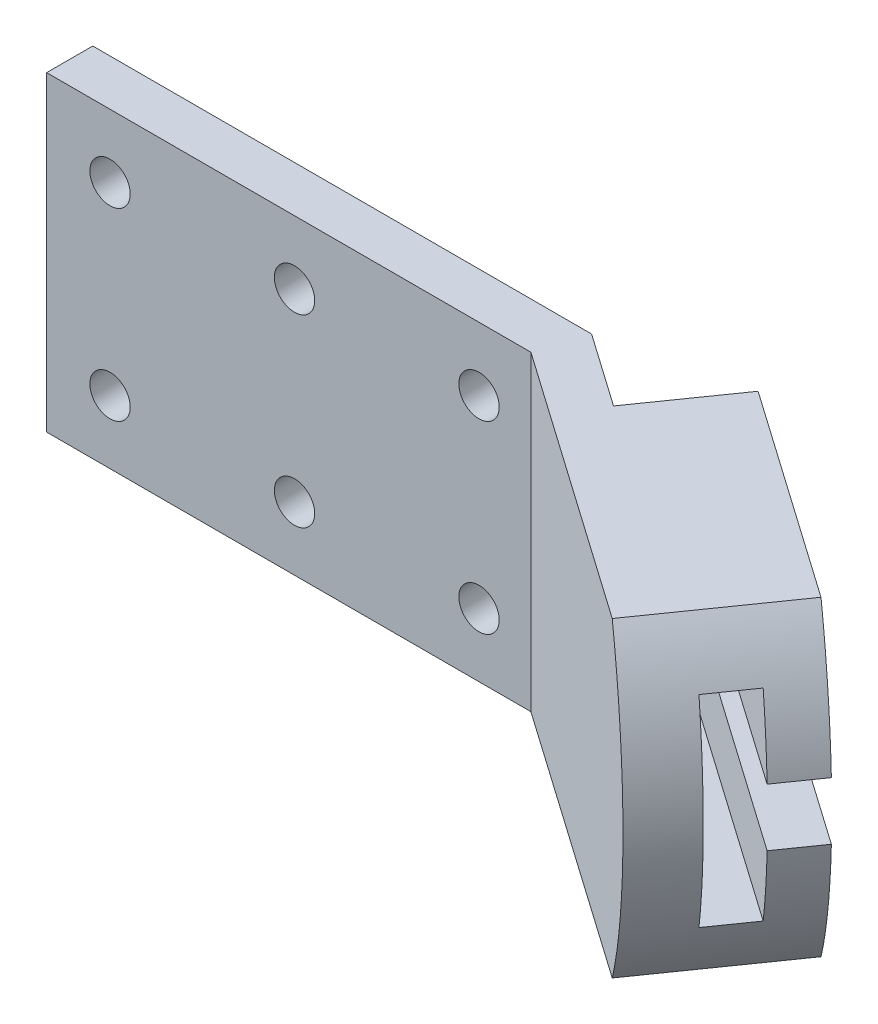
ISO-10303-21;
HEADER;
FILE_DESCRIPTION(('STEP AP214'),'2;1');
FILE_NAME('part.step','',(''),(''),'','','');
FILE_SCHEMA(('AUTOMOTIVE_DESIGN { 1 0 10303 214 1 1 1 1 }'));
ENDSEC;
DATA;
#1=APPLICATION_CONTEXT('core data for automotive mechanical design processes');
#2=APPLICATION_PROTOCOL_DEFINITION('international standard','automotive_design',2000,#1);
#3=PRODUCT_CONTEXT('',#1,'mechanical');
#4=PRODUCT('Part','Part','',(#3));
#5=PRODUCT_RELATED_PRODUCT_CATEGORY('part','',(#4));
#6=PRODUCT_DEFINITION_FORMATION('','',#4);
#7=PRODUCT_DEFINITION_CONTEXT('part definition',#1,'design');
#8=PRODUCT_DEFINITION('design','',#6,#7);
#9=PRODUCT_DEFINITION_SHAPE('','',#8);
#10=(LENGTH_UNIT() NAMED_UNIT(*) SI_UNIT(.MILLI.,.METRE.));
#11=(NAMED_UNIT(*) PLANE_ANGLE_UNIT() SI_UNIT($,.RADIAN.));
#12=(NAMED_UNIT(*) SI_UNIT($,.STERADIAN.) SOLID_ANGLE_UNIT());
#13=UNCERTAINTY_MEASURE_WITH_UNIT(LENGTH_MEASURE(1.E-05),#10,'distance_accuracy_value','');
#14=(GEOMETRIC_REPRESENTATION_CONTEXT(3) GLOBAL_UNCERTAINTY_ASSIGNED_CONTEXT((#13)) GLOBAL_UNIT_ASSIGNED_CONTEXT((#10,
#11,#12)) REPRESENTATION_CONTEXT('',''));
#15=CARTESIAN_POINT('',(0.,0.,0.));
#16=DIRECTION('',(0.,0.,1.));
#17=DIRECTION('',(1.,0.,0.));
#18=AXIS2_PLACEMENT_3D('',#15,#16,#17);
#19=CARTESIAN_POINT('',(152.157870223912,27.,15.9845152113043));
#20=DIRECTION('',(-0.573576436351047,0.,0.819152044288991));
#21=DIRECTION('',(0.819152044288991,0.,0.573576436351047));
#22=AXIS2_PLACEMENT_3D('',#19,#20,#21);
#23=PLANE('',#22);
#24=DIRECTION('',(0.81915204428899,0.,0.573576436351048));
#25=VECTOR('',#24,1.);
#26=CARTESIAN_POINT('',(78.0379109433139,5.,-35.9148390087672));
#27=LINE('',#26,#25);
#28=CARTESIAN_POINT('',(109.561963920884,5.,-13.8414594789501));
#29=VERTEX_POINT('',#28);
#30=CARTESIAN_POINT('',(151.960501419066,5.,15.8463160863439));
#31=VERTEX_POINT('',#30);
#32=EDGE_CURVE('E75',#29,#31,#27,.T.);
#33=ORIENTED_EDGE('',*,*,#32,.F.);
#34=DIRECTION('',(0.,-1.,0.));
#35=VECTOR('',#34,1.);
#36=CARTESIAN_POINT('',(109.561963920884,27.,-13.8414594789501));
#37=LINE('',#36,#35);
#38=CARTESIAN_POINT('',(109.561963920884,27.,-13.8414594789501));
#39=VERTEX_POINT('',#38);
#40=EDGE_CURVE('E259',#39,#29,#37,.T.);
#41=ORIENTED_EDGE('',*,*,#40,.F.);
#42=DIRECTION('',(-0.819152044288991,0.,-0.573576436351047));
#43=VECTOR('',#42,1.);
#44=CARTESIAN_POINT('',(152.157870223912,27.,15.9845152113043));
#45=LINE('',#44,#43);
#46=CARTESIAN_POINT('',(145.965877055795,27.,11.6488349184456));
#47=VERTEX_POINT('',#46);
#48=EDGE_CURVE('E222',#47,#39,#45,.T.);
#49=ORIENTED_EDGE('',*,*,#48,.F.);
#50=CARTESIAN_POINT('',(109.561963920884,0.,-13.8414594789502));
#51=DIRECTION('',(0.573576436351047,0.,-0.819152044288991));
#52=DIRECTION('',(-0.819152044288991,0.,-0.573576436351047));
#53=AXIS2_PLACEMENT_3D('',#50,#51,#52);
#54=CIRCLE('',#53,52.);
#55=EDGE_CURVE('E202',#47,#31,#54,.T.);
#56=ORIENTED_EDGE('',*,*,#55,.T.);
#57=EDGE_LOOP('',(#33,#41,#49,#56));
#58=FACE_BOUND('',#57,.T.);
#59=ADVANCED_FACE('F60',(#58),#23,.F.);
#60=CARTESIAN_POINT('',(99.2375880665653,27.,0.903277318251676));
#61=DIRECTION('',(0.81915204428899,0.,0.573576436351048));
#62=DIRECTION('',(0.573576436351048,0.,-0.81915204428899));
#63=AXIS2_PLACEMENT_3D('',#60,#61,#62);
#64=PLANE('',#63);
#65=DIRECTION('',(0.573576436351048,0.,-0.81915204428899));
#66=VECTOR('',#65,1.);
#67=CARTESIAN_POINT('',(67.0138225954348,5.,46.9235837455718));
#68=LINE('',#67,#66);
#69=CARTESIAN_POINT('',(104.973352430076,5.,-7.28824312463822));
#70=VERTEX_POINT('',#69);
#71=EDGE_CURVE('E193',#70,#29,#68,.T.);
#72=ORIENTED_EDGE('',*,*,#71,.F.);
#73=DIRECTION('',(0.,1.,0.));
#74=VECTOR('',#73,1.);
#75=CARTESIAN_POINT('',(104.973352430076,0.,-7.28824312463822));
#76=LINE('',#75,#74);
#77=CARTESIAN_POINT('',(104.973352430076,17.5,-7.28824312463822));
#78=VERTEX_POINT('',#77);
#79=EDGE_CURVE('E185',#70,#78,#76,.T.);
#80=ORIENTED_EDGE('',*,*,#79,.T.);
#81=DIRECTION('',(-0.573576436351048,0.,0.81915204428899));
#82=VECTOR('',#81,1.);
#83=CARTESIAN_POINT('',(67.0138225954348,17.5,46.9235837455718));
#84=LINE('',#83,#82);
#85=CARTESIAN_POINT('',(100.384740939267,17.5,-0.735026770326287));
#86=VERTEX_POINT('',#85);
#87=EDGE_CURVE('E173',#78,#86,#84,.T.);
#88=ORIENTED_EDGE('',*,*,#87,.T.);
#89=DIRECTION('',(0.,1.,0.));
#90=VECTOR('',#89,1.);
#91=CARTESIAN_POINT('',(100.384740939267,0.,-0.735026770326289));
#92=LINE('',#91,#90);
#93=CARTESIAN_POINT('',(100.384740939267,-17.5,-0.735026770326284));
#94=VERTEX_POINT('',#93);
#95=EDGE_CURVE('E182',#94,#86,#92,.T.);
#96=ORIENTED_EDGE('',*,*,#95,.F.);
#97=DIRECTION('',(-0.573576436351048,0.,0.81915204428899));
#98=VECTOR('',#97,1.);
#99=CARTESIAN_POINT('',(67.0138225954348,-17.5,46.9235837455718));
#100=LINE('',#99,#98);
#101=CARTESIAN_POINT('',(104.973352430076,-17.5,-7.28824312463823));
#102=VERTEX_POINT('',#101);
#103=EDGE_CURVE('E304',#102,#94,#100,.T.);
#104=ORIENTED_EDGE('',*,*,#103,.F.);
#105=DIRECTION('',(0.,1.,0.));
#106=VECTOR('',#105,1.);
#107=CARTESIAN_POINT('',(104.973352430076,0.,-7.28824312463822));
#108=LINE('',#107,#106);
#109=CARTESIAN_POINT('',(104.973352430076,-5.,-7.28824312463822));
#110=VERTEX_POINT('',#109);
#111=EDGE_CURVE('E299',#102,#110,#108,.T.);
#112=ORIENTED_EDGE('',*,*,#111,.T.);
#113=DIRECTION('',(0.573576436351048,0.,-0.81915204428899));
#114=VECTOR('',#113,1.);
#115=CARTESIAN_POINT('',(67.0138225954348,-5.,46.9235837455718));
#116=LINE('',#115,#114);
#117=CARTESIAN_POINT('',(109.561963920884,-5.,-13.8414594789501));
#118=VERTEX_POINT('',#117);
#119=EDGE_CURVE('E290',#110,#118,#116,.T.);
#120=ORIENTED_EDGE('',*,*,#119,.T.);
#121=CARTESIAN_POINT('',(109.561963920884,-27.,-13.8414594789501));
#122=VERTEX_POINT('',#121);
#123=EDGE_CURVE('E256',#118,#122,#37,.T.);
#124=ORIENTED_EDGE('',*,*,#123,.T.);
#125=DIRECTION('',(-0.573576436351048,0.,0.81915204428899));
#126=VECTOR('',#125,1.);
#127=CARTESIAN_POINT('',(99.2375880665653,-27.,0.903277318251676));
#128=LINE('',#127,#126);
#129=CARTESIAN_POINT('',(99.2375880665653,-27.,0.903277318251676));
#130=VERTEX_POINT('',#129);
#131=EDGE_CURVE('E238',#122,#130,#128,.T.);
#132=ORIENTED_EDGE('',*,*,#131,.T.);
#133=DIRECTION('',(0.,-1.,0.));
#134=VECTOR('',#133,1.);
#135=CARTESIAN_POINT('',(99.2375880665653,27.,0.903277318251676));
#136=LINE('',#135,#134);
#137=CARTESIAN_POINT('',(99.2375880665653,27.,0.903277318251676));
#138=VERTEX_POINT('',#137);
#139=EDGE_CURVE('E254',#138,#130,#136,.T.);
#140=ORIENTED_EDGE('',*,*,#139,.F.);
#141=DIRECTION('',(-0.573576436351048,0.,0.81915204428899));
#142=VECTOR('',#141,1.);
#143=CARTESIAN_POINT('',(99.2375880665653,27.,0.903277318251676));
#144=LINE('',#143,#142);
#145=EDGE_CURVE('E224',#39,#138,#144,.T.);
#146=ORIENTED_EDGE('',*,*,#145,.F.);
#147=ORIENTED_EDGE('',*,*,#40,.T.);
#148=EDGE_LOOP('',(#72,#80,#88,#96,#104,#112,#120,#124,#132,#140,#146,#147));
#149=FACE_BOUND('',#148,.T.);
#150=ADVANCED_FACE('F195',(#149),#64,.F.);
#151=CARTESIAN_POINT('',(78.5888363579276,0.,30.3927509126554));
#152=DIRECTION('',(0.573576436351047,0.,-0.819152044288991));
#153=DIRECTION('',(-0.819152044288991,0.,-0.573576436351047));
#154=AXIS2_PLACEMENT_3D('',#151,#152,#153);
#155=CYLINDRICAL_SURFACE('',#154,52.);
#156=CARTESIAN_POINT('',(151.960501419066,-5.,15.846316086344));
#157=VERTEX_POINT('',#156);
#158=CARTESIAN_POINT('',(145.965877055795,-27.,11.6488349184456));
#159=VERTEX_POINT('',#158);
#160=EDGE_CURVE('E207',#157,#159,#54,.T.);
#161=ORIENTED_EDGE('',*,*,#160,.F.);
#162=DIRECTION('',(0.573576436351047,0.,-0.819152044288991));
#163=VECTOR('',#162,1.);
#164=CARTESIAN_POINT('',(120.987373856109,-5.,60.0805264779494));
#165=LINE('',#164,#163);
#166=CARTESIAN_POINT('',(147.371889928258,-5.,22.3995324406559));
#167=VERTEX_POINT('',#166);
#168=EDGE_CURVE('E12',#157,#167,#165,.F.);
#169=ORIENTED_EDGE('',*,*,#168,.T.);
#170=CARTESIAN_POINT('',(104.973352430076,0.,-7.2882431246382));
#171=DIRECTION('',(-0.573576436351048,0.,0.81915204428899));
#172=DIRECTION('',(0.81915204428899,0.,0.573576436351048));
#173=AXIS2_PLACEMENT_3D('',#170,#171,#172);
#174=CIRCLE('',#173,52.);
#175=CARTESIAN_POINT('',(145.084627644528,-17.5,20.7979741477259));
#176=VERTEX_POINT('',#175);
#177=EDGE_CURVE('E64',#167,#176,#174,.F.);
#178=ORIENTED_EDGE('',*,*,#177,.T.);
#179=DIRECTION('',(0.573576436351047,0.,-0.819152044288991));
#180=VECTOR('',#179,1.);
#181=CARTESIAN_POINT('',(118.70011157238,-17.5,58.4789681850194));
#182=LINE('',#181,#180);
#183=CARTESIAN_POINT('',(140.49601615372,-17.5,27.3511905020379));
#184=VERTEX_POINT('',#183);
#185=EDGE_CURVE('E267',#184,#176,#182,.T.);
#186=ORIENTED_EDGE('',*,*,#185,.F.);
#187=CARTESIAN_POINT('',(100.384740939267,0.,-0.735026770326268));
#188=DIRECTION('',(-0.573576436351048,0.,0.81915204428899));
#189=DIRECTION('',(0.81915204428899,0.,0.573576436351048));
#190=AXIS2_PLACEMENT_3D('',#187,#188,#189);
#191=CIRCLE('',#190,52.);
#192=CARTESIAN_POINT('',(140.49601615372,17.5,27.3511905020378));
#193=VERTEX_POINT('',#192);
#194=EDGE_CURVE('E270',#193,#184,#191,.F.);
#195=ORIENTED_EDGE('',*,*,#194,.F.);
#196=DIRECTION('',(0.573576436351047,0.,-0.819152044288991));
#197=VECTOR('',#196,1.);
#198=CARTESIAN_POINT('',(118.70011157238,17.5,58.4789681850194));
#199=LINE('',#198,#197);
#200=CARTESIAN_POINT('',(145.084627644528,17.5,20.7979741477259));
#201=VERTEX_POINT('',#200);
#202=EDGE_CURVE('E264',#193,#201,#199,.T.);
#203=ORIENTED_EDGE('',*,*,#202,.T.);
#204=CARTESIAN_POINT('',(104.973352430076,0.,-7.2882431246382));
#205=DIRECTION('',(-0.573576436351048,0.,0.81915204428899));
#206=DIRECTION('',(0.81915204428899,0.,0.573576436351048));
#207=AXIS2_PLACEMENT_3D('',#204,#205,#206);
#208=CIRCLE('',#207,52.);
#209=CARTESIAN_POINT('',(147.371889928258,5.,22.3995324406559));
#210=VERTEX_POINT('',#209);
#211=EDGE_CURVE('E187',#201,#210,#208,.F.);
#212=ORIENTED_EDGE('',*,*,#211,.T.);
#213=DIRECTION('',(0.573576436351047,0.,-0.819152044288991));
#214=VECTOR('',#213,1.);
#215=CARTESIAN_POINT('',(120.987373856109,5.,60.0805264779494));
#216=LINE('',#215,#214);
#217=EDGE_CURVE('E204',#31,#210,#216,.F.);
#218=ORIENTED_EDGE('',*,*,#217,.F.);
#219=ORIENTED_EDGE('',*,*,#55,.F.);
#220=DIRECTION('',(0.573576436351047,0.,-0.819152044288991));
#221=VECTOR('',#220,1.);
#222=CARTESIAN_POINT('',(114.992749492838,27.,55.8830453100512));
#223=LINE('',#222,#221);
#224=CARTESIAN_POINT('',(131.052889710667,27.,32.9467880699594));
#225=VERTEX_POINT('',#224);
#226=EDGE_CURVE('E79',#225,#47,#223,.T.);
#227=ORIENTED_EDGE('',*,*,#226,.F.);
#228=CARTESIAN_POINT('',(94.6489765757569,0.,7.45649367256363));
#229=DIRECTION('',(0.573576436351047,0.,-0.819152044288991));
#230=DIRECTION('',(-0.819152044288991,0.,-0.573576436351047));
#231=AXIS2_PLACEMENT_3D('',#228,#229,#230);
#232=CIRCLE('',#231,52.);
#233=CARTESIAN_POINT('',(131.052889710667,-27.,32.9467880699594));
#234=VERTEX_POINT('',#233);
#235=EDGE_CURVE('E208',#225,#234,#232,.T.);
#236=ORIENTED_EDGE('',*,*,#235,.T.);
#237=DIRECTION('',(0.573576436351047,0.,-0.819152044288991));
#238=VECTOR('',#237,1.);
#239=CARTESIAN_POINT('',(114.992749492838,-27.,55.8830453100512));
#240=LINE('',#239,#238);
#241=EDGE_CURVE('E203',#234,#159,#240,.T.);
#242=ORIENTED_EDGE('',*,*,#241,.T.);
#243=EDGE_LOOP('',(#161,#169,#178,#186,#195,#203,#212,#218,#219,#227,#236,#242));
#244=FACE_BOUND('',#243,.T.);
#245=ADVANCED_FACE('F272',(#244),#155,.T.);
#246=CARTESIAN_POINT('',(137.244882878784,27.,37.2824683628181));
#247=DIRECTION('',(0.573576436351047,0.,-0.819152044288991));
#248=DIRECTION('',(-0.819152044288991,0.,-0.573576436351047));
#249=AXIS2_PLACEMENT_3D('',#246,#247,#248);
#250=PLANE('',#249);
#251=DIRECTION('',(0.819152044288991,0.,0.573576436351047));
#252=VECTOR('',#251,1.);
#253=CARTESIAN_POINT('',(137.244882878784,-27.,37.2824683628181));
#254=LINE('',#253,#252);
#255=CARTESIAN_POINT('',(84.,-27.,0.));
#256=VERTEX_POINT('',#255);
#257=EDGE_CURVE('E231',#256,#234,#254,.T.);
#258=ORIENTED_EDGE('',*,*,#257,.T.);
#259=ORIENTED_EDGE('',*,*,#235,.F.);
#260=DIRECTION('',(0.819152044288991,0.,0.573576436351047));
#261=VECTOR('',#260,1.);
#262=CARTESIAN_POINT('',(137.244882878784,27.,37.2824683628181));
#263=LINE('',#262,#261);
#264=CARTESIAN_POINT('',(84.,27.,0.));
#265=VERTEX_POINT('',#264);
#266=EDGE_CURVE('E220',#265,#225,#263,.T.);
#267=ORIENTED_EDGE('',*,*,#266,.F.);
#268=DIRECTION('',(0.,-1.,0.));
#269=VECTOR('',#268,1.);
#270=CARTESIAN_POINT('',(84.,27.,0.));
#271=LINE('',#270,#269);
#272=EDGE_CURVE('E211',#265,#256,#271,.T.);
#273=ORIENTED_EDGE('',*,*,#272,.T.);
#274=EDGE_LOOP('',(#258,#259,#267,#273));
#275=FACE_BOUND('',#274,.T.);
#276=ADVANCED_FACE('F350',(#275),#250,.F.);
#277=CARTESIAN_POINT('',(84.,27.,0.));
#278=DIRECTION('',(0.,0.,-1.));
#279=DIRECTION('',(-1.,0.,0.));
#280=AXIS2_PLACEMENT_3D('',#277,#278,#279);
#281=PLANE('',#280);
#282=CARTESIAN_POINT('',(75.,16.,0.));
#283=DIRECTION('',(0.,0.,-1.));
#284=DIRECTION('',(-1.,0.,0.));
#285=AXIS2_PLACEMENT_3D('',#282,#283,#284);
#286=CIRCLE('',#285,3.49999999999999);
#287=CARTESIAN_POINT('',(71.5,16.,0.));
#288=VERTEX_POINT('',#287);
#289=EDGE_CURVE('E330',#288,#288,#286,.F.);
#290=ORIENTED_EDGE('',*,*,#289,.F.);
#291=EDGE_LOOP('',(#290));
#292=FACE_BOUND('',#291,.T.);
#293=CARTESIAN_POINT('',(43.,-16.,0.));
#294=DIRECTION('',(0.,0.,-1.));
#295=DIRECTION('',(-1.,0.,0.));
#296=AXIS2_PLACEMENT_3D('',#293,#294,#295);
#297=CIRCLE('',#296,3.50000000000001);
#298=CARTESIAN_POINT('',(39.5,-16.,0.));
#299=VERTEX_POINT('',#298);
#300=EDGE_CURVE('E326',#299,#299,#297,.F.);
#301=ORIENTED_EDGE('',*,*,#300,.F.);
#302=EDGE_LOOP('',(#301));
#303=FACE_BOUND('',#302,.T.);
#304=CARTESIAN_POINT('',(43.,16.,0.));
#305=DIRECTION('',(0.,0.,-1.));
#306=DIRECTION('',(-1.,0.,0.));
#307=AXIS2_PLACEMENT_3D('',#304,#305,#306);
#308=CIRCLE('',#307,3.50000000000001);
#309=CARTESIAN_POINT('',(39.5,16.,0.));
#310=VERTEX_POINT('',#309);
#311=EDGE_CURVE('E312',#310,#310,#308,.F.);
#312=ORIENTED_EDGE('',*,*,#311,.F.);
#313=EDGE_LOOP('',(#312));
#314=FACE_BOUND('',#313,.T.);
#315=CARTESIAN_POINT('',(11.,-16.,0.));
#316=DIRECTION('',(0.,0.,-1.));
#317=DIRECTION('',(-1.,0.,0.));
#318=AXIS2_PLACEMENT_3D('',#315,#316,#317);
#319=CIRCLE('',#318,3.5);
#320=CARTESIAN_POINT('',(7.5,-16.,0.));
#321=VERTEX_POINT('',#320);
#322=EDGE_CURVE('E314',#321,#321,#319,.F.);
#323=ORIENTED_EDGE('',*,*,#322,.F.);
#324=EDGE_LOOP('',(#323));
#325=FACE_BOUND('',#324,.T.);
#326=CARTESIAN_POINT('',(75.,-16.,0.));
#327=DIRECTION('',(0.,0.,-1.));
#328=DIRECTION('',(-1.,0.,0.));
#329=AXIS2_PLACEMENT_3D('',#326,#327,#328);
#330=CIRCLE('',#329,3.49999999999999);
#331=CARTESIAN_POINT('',(71.5,-16.,0.));
#332=VERTEX_POINT('',#331);
#333=EDGE_CURVE('E340',#332,#332,#330,.F.);
#334=ORIENTED_EDGE('',*,*,#333,.F.);
#335=EDGE_LOOP('',(#334));
#336=FACE_BOUND('',#335,.T.);
#337=CARTESIAN_POINT('',(11.,16.,0.));
#338=DIRECTION('',(0.,0.,-1.));
#339=DIRECTION('',(-1.,0.,0.));
#340=AXIS2_PLACEMENT_3D('',#337,#338,#339);
#341=CIRCLE('',#340,3.5);
#342=CARTESIAN_POINT('',(7.5,16.,0.));
#343=VERTEX_POINT('',#342);
#344=EDGE_CURVE('E300',#343,#343,#341,.F.);
#345=ORIENTED_EDGE('',*,*,#344,.F.);
#346=EDGE_LOOP('',(#345));
#347=FACE_BOUND('',#346,.T.);
#348=DIRECTION('',(1.,0.,0.));
#349=VECTOR('',#348,1.);
#350=CARTESIAN_POINT('',(84.,-27.,0.));
#351=LINE('',#350,#349);
#352=CARTESIAN_POINT('',(0.,-27.,0.));
#353=VERTEX_POINT('',#352);
#354=EDGE_CURVE('E213',#353,#256,#351,.T.);
#355=ORIENTED_EDGE('',*,*,#354,.T.);
#356=ORIENTED_EDGE('',*,*,#272,.F.);
#357=DIRECTION('',(1.,0.,0.));
#358=VECTOR('',#357,1.);
#359=CARTESIAN_POINT('',(84.,27.,0.));
#360=LINE('',#359,#358);
#361=CARTESIAN_POINT('',(0.,27.,0.));
#362=VERTEX_POINT('',#361);
#363=EDGE_CURVE('E212',#362,#265,#360,.T.);
#364=ORIENTED_EDGE('',*,*,#363,.F.);
#365=DIRECTION('',(0.,-1.,0.));
#366=VECTOR('',#365,1.);
#367=CARTESIAN_POINT('',(0.,27.,0.));
#368=LINE('',#367,#366);
#369=EDGE_CURVE('E232',#362,#353,#368,.T.);
#370=ORIENTED_EDGE('',*,*,#369,.T.);
#371=EDGE_LOOP('',(#355,#356,#364,#370));
#372=FACE_BOUND('',#371,.T.);
#373=ADVANCED_FACE('F56',(#292,#303,#314,#325,#336,#347,#372),#281,.F.);
#374=ORIENTED_EDGE('',*,*,#123,.F.);
#375=DIRECTION('',(0.81915204428899,0.,0.573576436351048));
#376=VECTOR('',#375,1.);
#377=CARTESIAN_POINT('',(78.0379109433139,-5.,-35.9148390087672));
#378=LINE('',#377,#376);
#379=EDGE_CURVE('E197',#118,#157,#378,.T.);
#380=ORIENTED_EDGE('',*,*,#379,.T.);
#381=ORIENTED_EDGE('',*,*,#160,.T.);
#382=DIRECTION('',(-0.819152044288991,0.,-0.573576436351047));
#383=VECTOR('',#382,1.);
#384=CARTESIAN_POINT('',(152.157870223912,-27.,15.9845152113043));
#385=LINE('',#384,#383);
#386=EDGE_CURVE('E240',#159,#122,#385,.T.);
#387=ORIENTED_EDGE('',*,*,#386,.T.);
#388=EDGE_LOOP('',(#374,#380,#381,#387));
#389=FACE_BOUND('',#388,.T.);
#390=ADVANCED_FACE('F347',(#389),#23,.F.);
#391=CARTESIAN_POINT('',(86.5223903110319,27.,-8.));
#392=DIRECTION('',(-0.573576436351047,0.,0.819152044288991));
#393=DIRECTION('',(0.819152044288991,0.,0.573576436351047));
#394=AXIS2_PLACEMENT_3D('',#391,#392,#393);
#395=PLANE('',#394);
#396=DIRECTION('',(-0.819152044288991,0.,-0.573576436351047));
#397=VECTOR('',#396,1.);
#398=CARTESIAN_POINT('',(86.5223903110319,-27.,-8.));
#399=LINE('',#398,#397);
#400=CARTESIAN_POINT('',(86.5223903110319,-27.,-8.));
#401=VERTEX_POINT('',#400);
#402=EDGE_CURVE('E245',#130,#401,#399,.T.);
#403=ORIENTED_EDGE('',*,*,#402,.T.);
#404=DIRECTION('',(0.,-1.,0.));
#405=VECTOR('',#404,1.);
#406=CARTESIAN_POINT('',(86.5223903110319,27.,-8.));
#407=LINE('',#406,#405);
#408=CARTESIAN_POINT('',(86.5223903110319,27.,-8.));
#409=VERTEX_POINT('',#408);
#410=EDGE_CURVE('E252',#409,#401,#407,.T.);
#411=ORIENTED_EDGE('',*,*,#410,.F.);
#412=DIRECTION('',(-0.819152044288991,0.,-0.573576436351047));
#413=VECTOR('',#412,1.);
#414=CARTESIAN_POINT('',(86.5223903110319,27.,-8.));
#415=LINE('',#414,#413);
#416=EDGE_CURVE('E223',#138,#409,#415,.T.);
#417=ORIENTED_EDGE('',*,*,#416,.F.);
#418=ORIENTED_EDGE('',*,*,#139,.T.);
#419=EDGE_LOOP('',(#403,#411,#417,#418));
#420=FACE_BOUND('',#419,.T.);
#421=ADVANCED_FACE('F374',(#420),#395,.F.);
#422=CARTESIAN_POINT('',(0.,27.,-8.));
#423=DIRECTION('',(0.,0.,1.));
#424=DIRECTION('',(1.,0.,0.));
#425=AXIS2_PLACEMENT_3D('',#422,#423,#424);
#426=PLANE('',#425);
#427=CARTESIAN_POINT('',(75.,16.,-8.));
#428=DIRECTION('',(0.,0.,-1.));
#429=DIRECTION('',(-1.,0.,0.));
#430=AXIS2_PLACEMENT_3D('',#427,#428,#429);
#431=CIRCLE('',#430,3.49999999999999);
#432=CARTESIAN_POINT('',(71.5,16.,-8.));
#433=VERTEX_POINT('',#432);
#434=EDGE_CURVE('E323',#433,#433,#431,.T.);
#435=ORIENTED_EDGE('',*,*,#434,.F.);
#436=EDGE_LOOP('',(#435));
#437=FACE_BOUND('',#436,.T.);
#438=CARTESIAN_POINT('',(43.,-16.,-8.));
#439=DIRECTION('',(0.,0.,-1.));
#440=DIRECTION('',(-1.,0.,0.));
#441=AXIS2_PLACEMENT_3D('',#438,#439,#440);
#442=CIRCLE('',#441,3.50000000000001);
#443=CARTESIAN_POINT('',(39.5,-16.,-8.));
#444=VERTEX_POINT('',#443);
#445=EDGE_CURVE('E318',#444,#444,#442,.T.);
#446=ORIENTED_EDGE('',*,*,#445,.F.);
#447=EDGE_LOOP('',(#446));
#448=FACE_BOUND('',#447,.T.);
#449=CARTESIAN_POINT('',(43.,16.,-8.));
#450=DIRECTION('',(0.,0.,-1.));
#451=DIRECTION('',(-1.,0.,0.));
#452=AXIS2_PLACEMENT_3D('',#449,#450,#451);
#453=CIRCLE('',#452,3.50000000000001);
#454=CARTESIAN_POINT('',(39.5,16.,-8.));
#455=VERTEX_POINT('',#454);
#456=EDGE_CURVE('E313',#455,#455,#453,.T.);
#457=ORIENTED_EDGE('',*,*,#456,.F.);
#458=EDGE_LOOP('',(#457));
#459=FACE_BOUND('',#458,.T.);
#460=CARTESIAN_POINT('',(11.,-16.,-8.));
#461=DIRECTION('',(0.,0.,-1.));
#462=DIRECTION('',(-1.,0.,0.));
#463=AXIS2_PLACEMENT_3D('',#460,#461,#462);
#464=CIRCLE('',#463,3.5);
#465=CARTESIAN_POINT('',(7.5,-16.,-8.));
#466=VERTEX_POINT('',#465);
#467=EDGE_CURVE('E309',#466,#466,#464,.T.);
#468=ORIENTED_EDGE('',*,*,#467,.F.);
#469=EDGE_LOOP('',(#468));
#470=FACE_BOUND('',#469,.T.);
#471=CARTESIAN_POINT('',(75.,-16.,-8.));
#472=DIRECTION('',(0.,0.,-1.));
#473=DIRECTION('',(-1.,0.,0.));
#474=AXIS2_PLACEMENT_3D('',#471,#472,#473);
#475=CIRCLE('',#474,3.49999999999999);
#476=CARTESIAN_POINT('',(71.5,-16.,-8.));
#477=VERTEX_POINT('',#476);
#478=EDGE_CURVE('E329',#477,#477,#475,.T.);
#479=ORIENTED_EDGE('',*,*,#478,.F.);
#480=EDGE_LOOP('',(#479));
#481=FACE_BOUND('',#480,.T.);
#482=CARTESIAN_POINT('',(11.,16.,-8.));
#483=DIRECTION('',(0.,0.,-1.));
#484=DIRECTION('',(-1.,0.,0.));
#485=AXIS2_PLACEMENT_3D('',#482,#483,#484);
#486=CIRCLE('',#485,3.5);
#487=CARTESIAN_POINT('',(7.5,16.,-8.));
#488=VERTEX_POINT('',#487);
#489=EDGE_CURVE('E307',#488,#488,#486,.T.);
#490=ORIENTED_EDGE('',*,*,#489,.F.);
#491=EDGE_LOOP('',(#490));
#492=FACE_BOUND('',#491,.T.);
#493=DIRECTION('',(-1.,0.,0.));
#494=VECTOR('',#493,1.);
#495=CARTESIAN_POINT('',(0.,-27.,-8.));
#496=LINE('',#495,#494);
#497=CARTESIAN_POINT('',(0.,-27.,-8.));
#498=VERTEX_POINT('',#497);
#499=EDGE_CURVE('E242',#401,#498,#496,.T.);
#500=ORIENTED_EDGE('',*,*,#499,.T.);
#501=DIRECTION('',(0.,-1.,0.));
#502=VECTOR('',#501,1.);
#503=CARTESIAN_POINT('',(0.,27.,-8.));
#504=LINE('',#503,#502);
#505=CARTESIAN_POINT('',(0.,27.,-8.));
#506=VERTEX_POINT('',#505);
#507=EDGE_CURVE('E246',#506,#498,#504,.T.);
#508=ORIENTED_EDGE('',*,*,#507,.F.);
#509=DIRECTION('',(-1.,0.,0.));
#510=VECTOR('',#509,1.);
#511=CARTESIAN_POINT('',(0.,27.,-8.));
#512=LINE('',#511,#510);
#513=EDGE_CURVE('E230',#409,#506,#512,.T.);
#514=ORIENTED_EDGE('',*,*,#513,.F.);
#515=ORIENTED_EDGE('',*,*,#410,.T.);
#516=EDGE_LOOP('',(#500,#508,#514,#515));
#517=FACE_BOUND('',#516,.T.);
#518=ADVANCED_FACE('F367',(#437,#448,#459,#470,#481,#492,#517),#426,.F.);
#519=CARTESIAN_POINT('',(0.,27.,0.));
#520=DIRECTION('',(1.,0.,0.));
#521=DIRECTION('',(0.,0.,-1.));
#522=AXIS2_PLACEMENT_3D('',#519,#520,#521);
#523=PLANE('',#522);
#524=DIRECTION('',(0.,0.,1.));
#525=VECTOR('',#524,1.);
#526=CARTESIAN_POINT('',(0.,-27.,0.));
#527=LINE('',#526,#525);
#528=EDGE_CURVE('E217',#498,#353,#527,.T.);
#529=ORIENTED_EDGE('',*,*,#528,.T.);
#530=ORIENTED_EDGE('',*,*,#369,.F.);
#531=DIRECTION('',(0.,0.,1.));
#532=VECTOR('',#531,1.);
#533=CARTESIAN_POINT('',(0.,27.,0.));
#534=LINE('',#533,#532);
#535=EDGE_CURVE('E227',#506,#362,#534,.T.);
#536=ORIENTED_EDGE('',*,*,#535,.F.);
#537=ORIENTED_EDGE('',*,*,#507,.T.);
#538=EDGE_LOOP('',(#529,#530,#536,#537));
#539=FACE_BOUND('',#538,.T.);
#540=ADVANCED_FACE('F366',(#539),#523,.F.);
#541=CARTESIAN_POINT('',(0.,27.,0.));
#542=DIRECTION('',(0.,-1.,0.));
#543=DIRECTION('',(0.,0.,-1.));
#544=AXIS2_PLACEMENT_3D('',#541,#542,#543);
#545=PLANE('',#544);
#546=ORIENTED_EDGE('',*,*,#266,.T.);
#547=ORIENTED_EDGE('',*,*,#226,.T.);
#548=ORIENTED_EDGE('',*,*,#48,.T.);
#549=ORIENTED_EDGE('',*,*,#145,.T.);
#550=ORIENTED_EDGE('',*,*,#416,.T.);
#551=ORIENTED_EDGE('',*,*,#513,.T.);
#552=ORIENTED_EDGE('',*,*,#535,.T.);
#553=ORIENTED_EDGE('',*,*,#363,.T.);
#554=EDGE_LOOP('',(#546,#547,#548,#549,#550,#551,#552,#553));
#555=FACE_BOUND('',#554,.T.);
#556=ADVANCED_FACE('F361',(#555),#545,.F.);
#557=CARTESIAN_POINT('',(0.,-27.,0.));
#558=DIRECTION('',(0.,-1.,0.));
#559=DIRECTION('',(0.,0.,-1.));
#560=AXIS2_PLACEMENT_3D('',#557,#558,#559);
#561=PLANE('',#560);
#562=ORIENTED_EDGE('',*,*,#241,.F.);
#563=ORIENTED_EDGE('',*,*,#257,.F.);
#564=ORIENTED_EDGE('',*,*,#354,.F.);
#565=ORIENTED_EDGE('',*,*,#528,.F.);
#566=ORIENTED_EDGE('',*,*,#499,.F.);
#567=ORIENTED_EDGE('',*,*,#402,.F.);
#568=ORIENTED_EDGE('',*,*,#131,.F.);
#569=ORIENTED_EDGE('',*,*,#386,.F.);
#570=EDGE_LOOP('',(#562,#563,#564,#565,#566,#567,#568,#569));
#571=FACE_BOUND('',#570,.T.);
#572=ADVANCED_FACE('F360',(#571),#561,.T.);
#573=CARTESIAN_POINT('',(73.4492994525055,0.,-29.3616226544553));
#574=DIRECTION('',(-0.573576436351048,0.,0.81915204428899));
#575=DIRECTION('',(0.81915204428899,0.,0.573576436351048));
#576=AXIS2_PLACEMENT_3D('',#573,#574,#575);
#577=PLANE('',#576);
#578=DIRECTION('',(0.81915204428899,0.,0.573576436351048));
#579=VECTOR('',#578,1.);
#580=CARTESIAN_POINT('',(73.4492994525055,17.5,-29.3616226544553));
#581=LINE('',#580,#579);
#582=EDGE_CURVE('E172',#78,#201,#581,.T.);
#583=ORIENTED_EDGE('',*,*,#582,.F.);
#584=ORIENTED_EDGE('',*,*,#79,.F.);
#585=DIRECTION('',(0.81915204428899,0.,0.573576436351048));
#586=VECTOR('',#585,1.);
#587=CARTESIAN_POINT('',(73.4492994525055,5.,-29.3616226544553));
#588=LINE('',#587,#586);
#589=EDGE_CURVE('E189',#70,#210,#588,.T.);
#590=ORIENTED_EDGE('',*,*,#589,.T.);
#591=ORIENTED_EDGE('',*,*,#211,.F.);
#592=EDGE_LOOP('',(#583,#584,#590,#591));
#593=FACE_BOUND('',#592,.T.);
#594=ADVANCED_FACE('F183',(#593),#577,.T.);
#595=CARTESIAN_POINT('',(35.4897696178646,17.5,24.8502042157548));
#596=DIRECTION('',(0.,-1.,0.));
#597=DIRECTION('',(0.,0.,-1.));
#598=AXIS2_PLACEMENT_3D('',#595,#596,#597);
#599=PLANE('',#598);
#600=DIRECTION('',(0.81915204428899,0.,0.573576436351048));
#601=VECTOR('',#600,1.);
#602=CARTESIAN_POINT('',(68.8606879616971,17.5,-22.8084063001433));
#603=LINE('',#602,#601);
#604=EDGE_CURVE('E179',#86,#193,#603,.T.);
#605=ORIENTED_EDGE('',*,*,#604,.F.);
#606=ORIENTED_EDGE('',*,*,#87,.F.);
#607=ORIENTED_EDGE('',*,*,#582,.T.);
#608=ORIENTED_EDGE('',*,*,#202,.F.);
#609=EDGE_LOOP('',(#605,#606,#607,#608));
#610=FACE_BOUND('',#609,.T.);
#611=ADVANCED_FACE('F171',(#610),#599,.T.);
#612=CARTESIAN_POINT('',(68.8606879616971,0.,-22.8084063001433));
#613=DIRECTION('',(-0.573576436351048,0.,0.81915204428899));
#614=DIRECTION('',(0.81915204428899,0.,0.573576436351048));
#615=AXIS2_PLACEMENT_3D('',#612,#613,#614);
#616=PLANE('',#615);
#617=ORIENTED_EDGE('',*,*,#194,.T.);
#618=DIRECTION('',(0.81915204428899,0.,0.573576436351048));
#619=VECTOR('',#618,1.);
#620=CARTESIAN_POINT('',(68.8606879616971,-17.5,-22.8084063001433));
#621=LINE('',#620,#619);
#622=EDGE_CURVE('E288',#94,#184,#621,.T.);
#623=ORIENTED_EDGE('',*,*,#622,.F.);
#624=ORIENTED_EDGE('',*,*,#95,.T.);
#625=ORIENTED_EDGE('',*,*,#604,.T.);
#626=EDGE_LOOP('',(#617,#623,#624,#625));
#627=FACE_BOUND('',#626,.T.);
#628=ADVANCED_FACE('F460',(#627),#616,.F.);
#629=CARTESIAN_POINT('',(35.4897696178646,-17.5,24.8502042157548));
#630=DIRECTION('',(0.,-1.,0.));
#631=DIRECTION('',(0.,0.,-1.));
#632=AXIS2_PLACEMENT_3D('',#629,#630,#631);
#633=PLANE('',#632);
#634=ORIENTED_EDGE('',*,*,#185,.T.);
#635=DIRECTION('',(0.81915204428899,0.,0.573576436351048));
#636=VECTOR('',#635,1.);
#637=CARTESIAN_POINT('',(73.4492994525055,-17.5,-29.3616226544553));
#638=LINE('',#637,#636);
#639=EDGE_CURVE('E281',#102,#176,#638,.T.);
#640=ORIENTED_EDGE('',*,*,#639,.F.);
#641=ORIENTED_EDGE('',*,*,#103,.T.);
#642=ORIENTED_EDGE('',*,*,#622,.T.);
#643=EDGE_LOOP('',(#634,#640,#641,#642));
#644=FACE_BOUND('',#643,.T.);
#645=ADVANCED_FACE('F458',(#644),#633,.F.);
#646=CARTESIAN_POINT('',(73.4492994525055,0.,-29.3616226544553));
#647=DIRECTION('',(-0.573576436351048,0.,0.81915204428899));
#648=DIRECTION('',(0.81915204428899,0.,0.573576436351048));
#649=AXIS2_PLACEMENT_3D('',#646,#647,#648);
#650=PLANE('',#649);
#651=DIRECTION('',(0.81915204428899,0.,0.573576436351048));
#652=VECTOR('',#651,1.);
#653=CARTESIAN_POINT('',(73.4492994525055,-5.,-29.3616226544553));
#654=LINE('',#653,#652);
#655=EDGE_CURVE('E278',#110,#167,#654,.T.);
#656=ORIENTED_EDGE('',*,*,#655,.F.);
#657=ORIENTED_EDGE('',*,*,#111,.F.);
#658=ORIENTED_EDGE('',*,*,#639,.T.);
#659=ORIENTED_EDGE('',*,*,#177,.F.);
#660=EDGE_LOOP('',(#656,#657,#658,#659));
#661=FACE_BOUND('',#660,.T.);
#662=ADVANCED_FACE('F276',(#661),#650,.T.);
#663=CARTESIAN_POINT('',(35.4897696178646,-5.,24.8502042157548));
#664=DIRECTION('',(0.,1.,0.));
#665=DIRECTION('',(0.,0.,1.));
#666=AXIS2_PLACEMENT_3D('',#663,#664,#665);
#667=PLANE('',#666);
#668=ORIENTED_EDGE('',*,*,#379,.F.);
#669=ORIENTED_EDGE('',*,*,#119,.F.);
#670=ORIENTED_EDGE('',*,*,#655,.T.);
#671=ORIENTED_EDGE('',*,*,#168,.F.);
#672=EDGE_LOOP('',(#668,#669,#670,#671));
#673=FACE_BOUND('',#672,.T.);
#674=ADVANCED_FACE('F284',(#673),#667,.T.);
#675=CARTESIAN_POINT('',(35.4897696178646,5.,24.8502042157548));
#676=DIRECTION('',(0.,1.,0.));
#677=DIRECTION('',(0.,0.,1.));
#678=AXIS2_PLACEMENT_3D('',#675,#676,#677);
#679=PLANE('',#678);
#680=ORIENTED_EDGE('',*,*,#217,.T.);
#681=ORIENTED_EDGE('',*,*,#589,.F.);
#682=ORIENTED_EDGE('',*,*,#71,.T.);
#683=ORIENTED_EDGE('',*,*,#32,.T.);
#684=EDGE_LOOP('',(#680,#681,#682,#683));
#685=FACE_BOUND('',#684,.T.);
#686=ADVANCED_FACE('F400',(#685),#679,.F.);
#687=CARTESIAN_POINT('',(11.,16.,9.89949493661168));
#688=DIRECTION('',(0.,0.,-1.));
#689=DIRECTION('',(-1.,0.,0.));
#690=AXIS2_PLACEMENT_3D('',#687,#688,#689);
#691=CYLINDRICAL_SURFACE('',#690,3.5);
#692=ORIENTED_EDGE('',*,*,#344,.T.);
#693=EDGE_LOOP('',(#692));
#694=FACE_BOUND('',#693,.T.);
#695=ORIENTED_EDGE('',*,*,#489,.T.);
#696=EDGE_LOOP('',(#695));
#697=FACE_BOUND('',#696,.T.);
#698=ADVANCED_FACE('F398',(#694,#697),#691,.F.);
#699=CARTESIAN_POINT('',(75.,-16.,9.89949493661168));
#700=DIRECTION('',(0.,0.,-1.));
#701=DIRECTION('',(-1.,0.,0.));
#702=AXIS2_PLACEMENT_3D('',#699,#700,#701);
#703=CYLINDRICAL_SURFACE('',#702,3.49999999999999);
#704=ORIENTED_EDGE('',*,*,#333,.T.);
#705=EDGE_LOOP('',(#704));
#706=FACE_BOUND('',#705,.T.);
#707=ORIENTED_EDGE('',*,*,#478,.T.);
#708=EDGE_LOOP('',(#707));
#709=FACE_BOUND('',#708,.T.);
#710=ADVANCED_FACE('F342',(#706,#709),#703,.F.);
#711=CARTESIAN_POINT('',(11.,-16.,9.89949493661168));
#712=DIRECTION('',(0.,0.,-1.));
#713=DIRECTION('',(-1.,0.,0.));
#714=AXIS2_PLACEMENT_3D('',#711,#712,#713);
#715=CYLINDRICAL_SURFACE('',#714,3.5);
#716=ORIENTED_EDGE('',*,*,#322,.T.);
#717=EDGE_LOOP('',(#716));
#718=FACE_BOUND('',#717,.T.);
#719=ORIENTED_EDGE('',*,*,#467,.T.);
#720=EDGE_LOOP('',(#719));
#721=FACE_BOUND('',#720,.T.);
#722=ADVANCED_FACE('F432',(#718,#721),#715,.F.);
#723=CARTESIAN_POINT('',(43.,16.,9.89949493661168));
#724=DIRECTION('',(0.,0.,-1.));
#725=DIRECTION('',(-1.,0.,0.));
#726=AXIS2_PLACEMENT_3D('',#723,#724,#725);
#727=CYLINDRICAL_SURFACE('',#726,3.50000000000001);
#728=ORIENTED_EDGE('',*,*,#311,.T.);
#729=EDGE_LOOP('',(#728));
#730=FACE_BOUND('',#729,.T.);
#731=ORIENTED_EDGE('',*,*,#456,.T.);
#732=EDGE_LOOP('',(#731));
#733=FACE_BOUND('',#732,.T.);
#734=ADVANCED_FACE('F438',(#730,#733),#727,.F.);
#735=CARTESIAN_POINT('',(43.,-16.,9.89949493661168));
#736=DIRECTION('',(0.,0.,-1.));
#737=DIRECTION('',(-1.,0.,0.));
#738=AXIS2_PLACEMENT_3D('',#735,#736,#737);
#739=CYLINDRICAL_SURFACE('',#738,3.50000000000001);
#740=ORIENTED_EDGE('',*,*,#300,.T.);
#741=EDGE_LOOP('',(#740));
#742=FACE_BOUND('',#741,.T.);
#743=ORIENTED_EDGE('',*,*,#445,.T.);
#744=EDGE_LOOP('',(#743));
#745=FACE_BOUND('',#744,.T.);
#746=ADVANCED_FACE('F444',(#742,#745),#739,.F.);
#747=CARTESIAN_POINT('',(75.,16.,9.89949493661168));
#748=DIRECTION('',(0.,0.,-1.));
#749=DIRECTION('',(-1.,0.,0.));
#750=AXIS2_PLACEMENT_3D('',#747,#748,#749);
#751=CYLINDRICAL_SURFACE('',#750,3.49999999999999);
#752=ORIENTED_EDGE('',*,*,#289,.T.);
#753=EDGE_LOOP('',(#752));
#754=FACE_BOUND('',#753,.T.);
#755=ORIENTED_EDGE('',*,*,#434,.T.);
#756=EDGE_LOOP('',(#755));
#757=FACE_BOUND('',#756,.T.);
#758=ADVANCED_FACE('F448',(#754,#757),#751,.F.);
#759=CLOSED_SHELL('',(#59,#150,#245,#276,#373,#390,#421,#518,#540,#556,#572,#594,#611,#628,#645,
#662,#674,#686,#698,#710,#722,#734,#746,#758));
#760=MANIFOLD_SOLID_BREP('B2',#759);
#761=ADVANCED_BREP_SHAPE_REPRESENTATION('',(#18,#760),#14);
#762=SHAPE_DEFINITION_REPRESENTATION(#9,#761);
ENDSEC;
END-ISO-10303-21;
